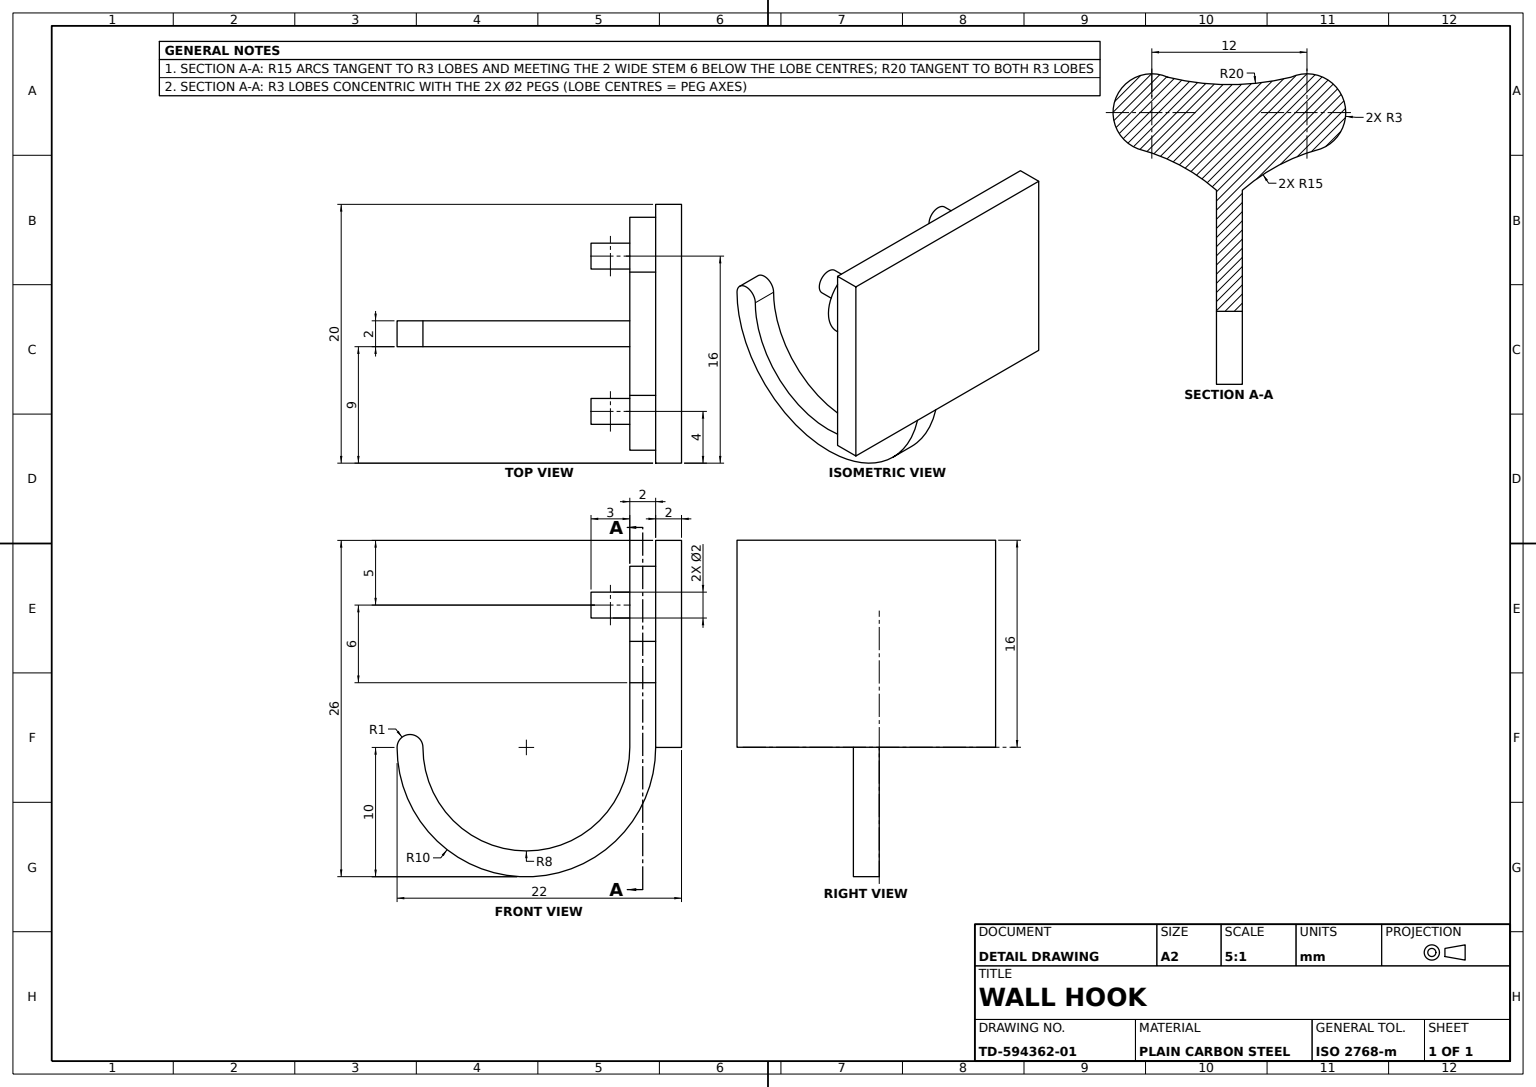
SolidWorks part; units mm, degrees
material "Plain Carbon Steel"
ref_plane "Front Plane" through (0, 0, 0) normal (0, 0, 1) x (1, 0, 0)
ref_plane "Top Plane" through (0, 0, 0) normal (0, 1, 0) x (1, 0, 0)
ref_plane "Right Plane" through (0, 0, 0) normal (1, 0, 0) x (0, 0, -1)
sketch "Back Plate Sketch" plane through (0, 0, 0) normal (0, 0, 1) x (1, 0, 0)
  line L1 (-10, -8) -> (10, -8)
  line L2 (-10, -8) -> (-10, 8)
  line L3 (-10, 8) -> (10, 8)
  line L4 (10, -8) -> (10, 8)
  line L5 (-10, -8) -> (10, 8) construction
  line L6 (-10, 8) -> (10, -8) construction
  point P0 (0, 0)
  dimension "D1" = 16
  dimension "D2" = 20
extrude "Back Plate 16x20x2" add sketch "Back Plate Sketch" along normal blind 2
sketch "Bracket Profile Sketch" plane through (0, 0, 2) normal (0, 0, 1) x (1, 0, 0)
  line L0 (10, 8) -> (-10, 8) construction
  line L1 (0, 4.7723) -> (0, -5.6217) construction
  line L2 (-10, -8) -> (10, -8) construction
  line L4 (-1, -3) -> (-1, -8)
  line L5 (-1, -8) -> (1, -8)
  line L6 (1, -3) -> (1, -8)
  line L7 (10, -8) -> (10, 8) construction
  circle A0 centre (-6, 3) radius 1
  circle A1 centre (6, 3) radius 1
  arc A2 (-4.7634, 5.7333) -> (-7.0634, 0.1948) centre (-6, 3) ccw
  arc A3 (7.0634, 0.1948) -> (4.7634, 5.7333) centre (6, 3) ccw
  arc A4 (-4.7634, 5.7333) -> (4.7634, 5.7333) centre (0, 25.1577) ccw
  arc A5 (-7.0634, 0.1948) -> (-1, -3) centre (-10.839, -14.3222) cw
  arc A6 (7.0634, 0.1948) -> (1, -3) centre (10.839, -14.3222) ccw
  dimension "D1" = 2
  dimension "D4" = 6
  dimension "D5" = 0.839
  dimension "D6" = 20
  dimension "D9" = 15
  dimension "D2" = 5
  dimension "D3" = 6
  dimension "D7" = 2
  dimension "D8" = 5
  dimension "D10" = 5.2366
extrude "Hook Bracket" add sketch "Bracket Profile Sketch" along normal blind 2
sketch "Pin Circles Sketch" plane through (0, 0, 2) normal (0, 0, 1) x (1, 0, 0)
  circle A1 centre (-6, 3) radius 1
  circle A2 centre (-6, 3) radius 1
  circle A3 centre (6, 3) radius 1
  circle A4 centre (6, 3) radius 1
  dimension "D1" = 0
  dimension "D2" = 0
extrude "Mounting Pins 2x" add sketch "Pin Circles Sketch" along normal blind 5
sketch "Hook Path Sketch" plane through (0, 0, 0) normal (1, 0, 0) x (0, 0, -1)
  line L2 (-4, -8) -> (-2, -8) construction
  arc A0 (-3, -8) -> (-21, -8) centre (-12, -8) cw
  dimension "D1" = 9
  dimension "D2" = 18
sketch "Hook Section Sketch" plane through (0, -8, 0) normal (0, -1, 0) x (1, 0, 0)
  line L0 (-1, 2) -> (1, 2)
  line L8 (-10, 0) -> (10, 0)
  line L9 (10, 0) -> (10, 2)
  line L10 (10, 2) -> (1, 2)
  line L11 (1, 2) -> (1, 4)
  line L12 (1, 4) -> (-1, 4)
  line L13 (-1, 4) -> (-1, 2)
  line L14 (-1, 2) -> (-10, 2)
  line L15 (-10, 2) -> (-10, 0)
  line L19 (1, 2) -> (1, 4)
  line L20 (1, 4) -> (-1, 4)
  line L21 (-1, 4) -> (-1, 2)
  dimension "D1" = 0
sweep "Hook Arm Sweep" add profiles "Hook Section Sketch" path "Hook Path Sketch"
sketch "Hook Tip Sketch" plane through (-1, 0, 0) normal (-1, 0, 0) x (0, 0, 1)
  line L0 (20, -8) -> (22, -8) construction
  line L1 (20, -8) -> (22, -8)
  arc A0 (22, -8) -> (20, -8) centre (21, -8) ccw
extrude "Hook Tip" add sketch "Hook Tip Sketch" against normal blind 2
